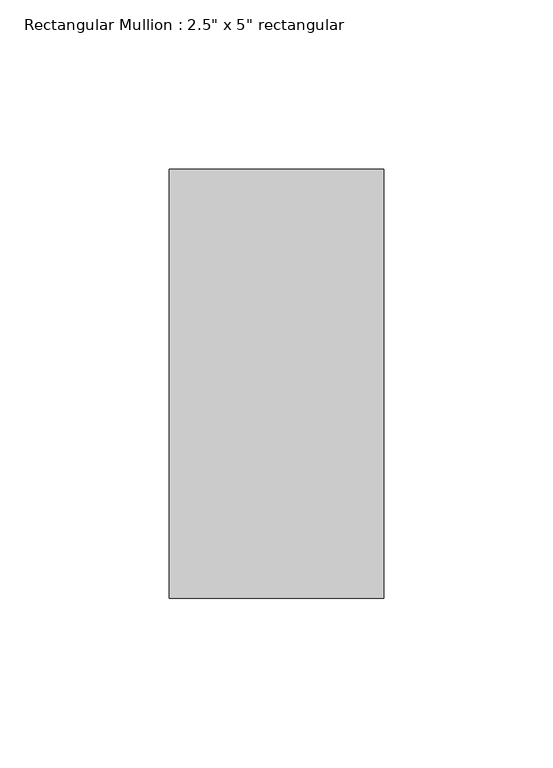
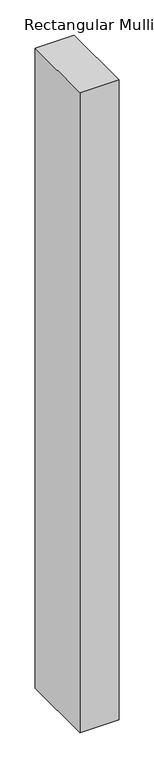
"""IFC4 building model written with IfcOpenShell, lengths in millimetres: member geometry."""

from ifc_helpers import new_model, si_unit, frame, origin, place, context, project, spatial, polyline, outline, extrude, source, transform, mapped, element, save


def member_8897803d(model_context):
    return source(origin(), model_context, "Body", "SweptSolid", [
        extrude(outline(polyline([(0.0, 63.5), (0.0, -63.5), (-63.5, -63.5), (-63.5, 63.5), (0.0, 63.5)])), frame((0.0, 0.0, -1104.9), z_axis=(0.0, 0.0, 1.0), x_axis=(1.0, 0.0, 0.0)), (0.0, 0.0, 1.0), 1104.9),
    ])


if __name__ == "__main__":
    model = new_model("IFC4")
    model_context = context("Model", 3, world=origin())
    ifc_project = project(units=[si_unit("LENGTHUNIT", "METRE", prefix="MILLI")], contexts=[model_context])
    site = spatial("IfcSite", under=ifc_project)
    building = spatial("IfcBuilding", under=site)
    placement = place(None, origin())
    member_shape = member_8897803d(model_context)
    element("IfcMember", 1, ObjectType="Rectangular Mullion : 2.5\" x 5\" rectangular", at=placement, inside=building, context=model_context, shape_type="MappedRepresentation", body=[
        mapped(member_shape, transform((0.0, 0.0, 0.0), x_axis=(1.0, 0.0, 0.0), y_axis=(0.0, 1.0, 0.0), z_axis=(0.0, 0.0, 1.0))),
    ])
    save(model, "model.ifc")

# Revit data of these elements
# Type "Rectangular Mullion : 2.5\" x 5\" rectangular"
#   built-in parameter 1007304 = 0.416667 (stored number, unit not read)
#   built-in parameter 1007301 = 0.104167 (stored number, unit not read)
#   built-in parameter 1007300 = 0.104167 (stored number, unit not read)
# Element 1 (IfcMember, "Rectangular Mullion : 2.5\" x 5\" rectangular")
#   Materials on its faces: "Iron, Ductile"
# Materials
#   "Iron, Ductile": class "Metal", colour RGB 0 0 0, transparency 0, Description = "Ductile cast iron", Cost = 0
